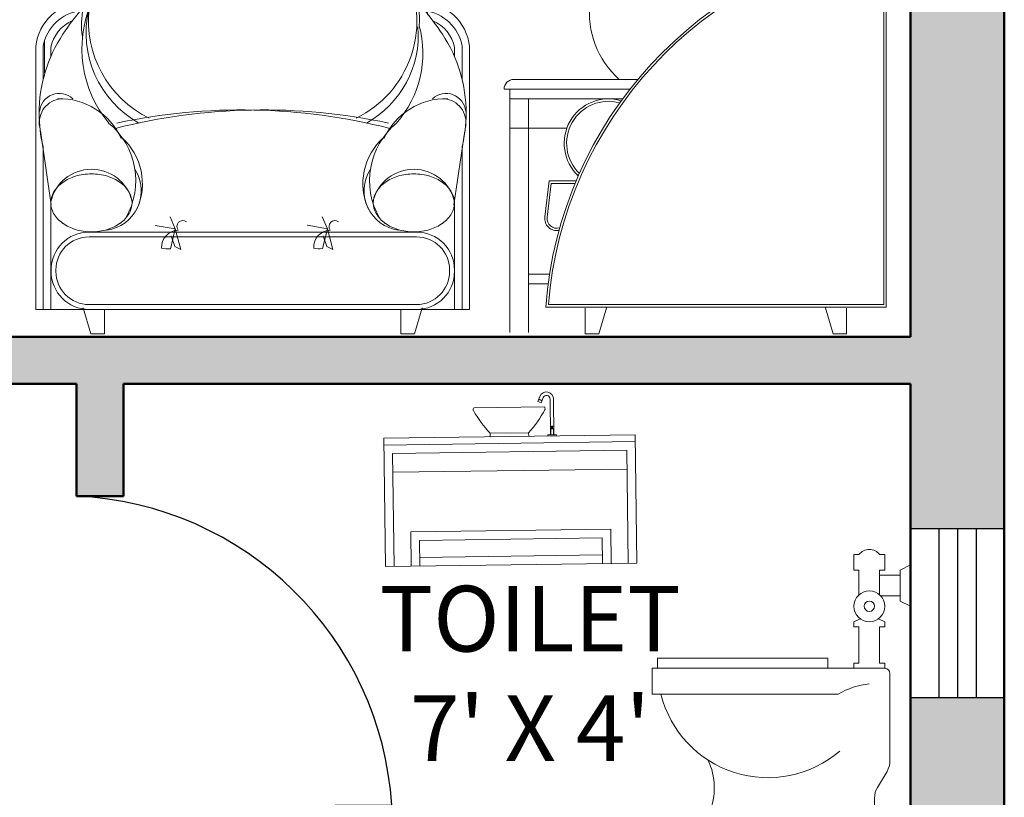
# Model space of a CAD drawing. Units: inches. Extents: x 1771 to 3025, y 319 to 889.
# Tile 21 of 35: x 2456 to 2561, y 621 to 703. Entities that reach past the tile are written whole.
import ezdxf

# ---------------------------------------------------------------- set-up
doc = ezdxf.new("R2010")
doc.units = ezdxf.units.IN
doc.header["$MEASUREMENT"] = 0
doc.set_wipeout_variables(frame=1)
for name, color, linetype, lineweight in [('A-AREA-IDEN', 241, 'Continuous', 25), ('A-DOOR', 4, 'Continuous', 25), ('A-FLOR-FIXT', 8, 'Continuous', 18), ('A-FURN', 8, 'Continuous', 18), ('A-GLAZ', 40, 'Continuous', 25), ('A-WALL', 7, 'Continuous', 50), ('A-WALL-PATT', 254, 'Continuous', 13)]:
    doc.layers.add(name, color=color, linetype=linetype, lineweight=lineweight)
doc.styles.get("Standard").update_dxf_attribs({"font": 'arial.ttf'})

# ---------------------------------------------------------------- blocks, each defined once
blk = doc.blocks.new('A$C425441F1')
for points in [[(1639.3, 0), (1667.3, 0), (1667.3, 55.3), (1748.6, 55.3), (1748.6, 807.4), (1761.1, 860.7), (1735.7, 880.7), (1703.4, 883.3), (1675.8, 879.6), (1656.2, 873.5), (1635.2, 863.3), (1619.6, 852.6), (1605.1, 839.5), (1596.7, 829.9), (1583.2, 810), (1573.2, 788.1), (1567.6, 767.7), (1566.5, 761.6), (1541.6, 750.9), (1510.7, 736.6), (1488.3, 725.3), (1464.5, 712.2), (1433.4, 693.6), (1409.1, 677.8), (1389.7, 664.2), (1388.2, 683.8), (1383.3, 700), (1376.2, 712), (1365.5, 723.2), (1352, 731.8), (1342.1, 735.4), (1331.7, 738.6), (1325, 742.7), (1317.7, 750.9), (1314.2, 758.8), (1312.9, 767.9), (1315.6, 780.8), (1321.1, 788.9), (1323.4, 793.7), (1323.6, 797.2), (1323.1, 800), (1320.5, 804.5), (1317.8, 806.7), (1317.8, 807.1), (1478.8, 807.1), (1345.8, 1080.7), (1177.3, 1080.7), (1044.3, 807.1), (1211.1, 807.1), (1211.1, 806.7), (1207.8, 803.9), (1205.8, 800.4), (1205.1, 796.3), (1207.6, 788.9), (1211.4, 783.4), (1213.5, 778.7), (1215.3, 769.8), (1215.1, 763.9), (1214.1, 759), (1208.8, 748.5), (1201.9, 741.7), (1195.3, 738), (1185.9, 735.4), (1176, 731.7), (1166.8, 726.4), (1159.9, 720.8), (1156.8, 717.7), (1149.3, 708.1), (1145.7, 701.6), (1143.6, 696.9), (1138.7, 669.7), (1138.7, 651.6), (1140.7, 631.8), (1142.6, 621.6), (1148.5, 600.5), (1162.8, 569), (1176.9, 547.8), (1188.6, 534.2), (1200, 523), (983, 523), (977.7, 522.3), (971.8, 519.6), (965.5, 512.8), (963.3, 506.8), (963, 503), (974.8, 503), (974.8, 3), (1013, 3), (1013, 103), (1053.6, 103), (1052.7, 96.1), (1051.6, 86.5), (1049.3, 63.6), (1048.6, 55.3), (1130.1, 55.3), (1130.1, 0), (1157.9, 0), (1174.1, 55.3), (1623.1, 55.6)], [(778.6, 0), (750.6, 0), (750.6, 50.4), (141.4, 50.4), (141.4, 0), (113.4, 0), (98.1, 50.4), (0, 50.4), (0, 590.4), (3.6, 609.1), (14.7, 633.7), (36.6, 658.7), (60.6, 673.3), (86.6, 680.5), (100.5, 681.5), (107.8, 698), (118.3, 717), (136.4, 751.3), (159.1, 779.5), (188.4, 803.6), (213.2, 817.4), (239.4, 827.1), (258.7, 831.4), (276, 833.4), (301.1, 842.1), (332.2, 850.9), (368.4, 858.6), (403.3, 863.5), (432.7, 865.8), (472.6, 866.2), (499.3, 864.8), (525, 862.1), (551.9, 857.9), (572.9, 853.6), (591.1, 849.1), (612.6, 842.8), (648, 830.4), (661.5, 823.7), (679.5, 815.2), (707.5, 798.2), (726.7, 783.3), (755.4, 754.4), (773.7, 729.8), (788.1, 704.9), (796.6, 686.1), (798.5, 681.2), (818, 677.9), (833.5, 672.3), (851.7, 661.6), (864.4, 650.3), (878.3, 632.1), (887.5, 611.7), (891.4, 595.2), (892, 590.4), (892, 50.4), (793.9, 50.4)]]:
    blk.add_wipeout(points)
for p, q in [((1044.3, 807.1), (1177.3, 1080.7)), ((1177.3, 1080.7), (1044.3, 807.1)), ((1177.3, 1080.7), (1345.8, 1080.7)), ((1345.8, 1080.7), (1177.3, 1080.7)), ((1345.8, 1080.7), (1478.8, 807.1)), ((1478.8, 807.1), (1345.8, 1080.7)), ((1188.8, 1068), (1069.3, 827.4)), ((1201.1, 1068), (1081.6, 827.4)), ((1211.2, 1068), (1091.7, 827.4)), ((1223.5, 1068), (1104, 827.4)), ((1230.5, 1068), (1110.9, 827.4)), ((1242.8, 1068), (1123.2, 827.4)), ((1171, 1067.8), (1351.9, 1067.8)), ((1299.6, 1068), (1419.2, 827.4)), ((1311.9, 1068), (1431.5, 827.4)), ((1322, 1068), (1441.5, 827.4)), ((1334.3, 1068), (1453.8, 827.4)), ((1733.6, 876.1), (1755.5, 858.7)), ((1735.7, 880.7), (1761.1, 860.7)), ((1744.1, 810.1), (1755.5, 858.7)), ((1748.6, 807.4), (1761.1, 860.7)), ((1053.8, 826.7), (1469.3, 826.7)), ((1478.8, 807.1), (1044.3, 807.1)), ((1044.3, 807.1), (1478.8, 807.1)), ((1205.6, 800), (1323.1, 800)), ((1211, 806.7), (1317.8, 806.7)), ((1743.6, 60.3), (1743.6, 805)), ((1748.6, 55.3), (1748.6, 807.4)), ((0, 590.4), (0, 50.4)), ((15, 591.1), (15, 521.6)), ((18.2, 603.6), (18.2, 536.8)), ((31, 569.9), (31, 588.4)), ((861, 569.9), (861, 588.4)), ((877, 591.1), (877, 521.6)), ((892, 590.4), (892, 50.4)), ((1238.2, 523), (983, 523)), ((1222, 503), (963, 503)), ((974.8, 3), (974.8, 503)), ((1206.8, 483), (974.8, 483)), ((1013, 3), (1013, 483)), ((10, 417.4), (32, 265.4)), ((882, 417.4), (860, 265.4)), ((1092.2, 423), (974.8, 423)), ((15, 385.1), (15, 50.4)), ((877, 385.1), (877, 50.4)), ((1055.6, 314.3), (1046.6, 240.3)), ((1060.1, 309.3), (1051.6, 239.7)), ((1111.1, 314.3), (1055.6, 314.3)), ((1109, 309.3), (1060.1, 309.3)), ((31, 50.4), (31, 272.3)), ((861, 50.4), (861, 272.3)), ((245.5, 223.1), (286.9, 216)), ((276.3, 240.8), (286.9, 216)), ((558.4, 223.2), (599.9, 216.1)), ((589.2, 240.9), (599.9, 216.1)), ((108.8, 209.4), (790.1, 209.4)), ((109.6, 209.4), (783, 209.4)), ((286.9, 216), (276.9, 175.2)), ((286.9, 216), (298.3, 173.5)), ((599.9, 216.1), (589.8, 175.3)), ((599.9, 216.1), (611.2, 173.6)), ((109.6, 199.4), (783, 199.4)), ((285.7, 179.9), (278.3, 201.7)), ((598.7, 180), (591.2, 201.8)), ((298.3, 173.5), (285.7, 179.9)), ((611.2, 173.6), (598.7, 180)), ((31.6, 128.4), (31.6, 131.4)), ((41.6, 128.4), (41.6, 131.4)), ((851, 131.4), (851, 128.4)), ((861, 131.4), (861, 128.4)), ((1056.5, 123), (1013, 123)), ((1053.6, 103), (1013, 103)), ((0, 50.4), (892, 50.4)), ((113.4, 0), (97.2, 53.4)), ((783, 60.4), (109.6, 60.4)), ((783, 50.4), (109.6, 50.4)), ((141.4, 50.4), (141.4, 0)), ((750.6, 50.4), (750.6, 0)), ((778.6, 0), (794.8, 53.4)), ((1048.6, 55.3), (1748.6, 55.3)), ((1054, 60.3), (1743.6, 60.3)), ((1129.9, 52.6), (1129.9, 0)), ((1157.9, 0), (1174.2, 55.6)), ((1639.3, 0), (1623.1, 55.6)), ((1667.3, 52.6), (1667.3, 0)), ((141.4, 0), (113.4, 0)), ((750.6, 0), (778.6, 0)), ((1129.9, 0), (1157.9, 0)), ((1667.3, 0), (1639.3, 0))]:
    blk.add_line(p, q)
for centre, radius, start, end in [((1708.4, 739.8), 143.6, 79.0486, 171.2543), ((1708.4, 739.8), 138.6, 79.5487, 170.0411), ((458.1, 348.7), 517.8, 68.4843, 110.5916), ((458.1, 348.7), 512.8, 68.4843, 110.5916), ((289.3, 651.4), 182.6, 93.9855, 176.965), ((563, 591.9), 251.9, 14.3659, 71.2419), ((289.3, 651.4), 177.6, 93.9855, 170.8791), ((563, 591.9), 246.9, 17.5917, 71.2419), ((1873.1, -6.5), 826.8, 98.9741, 175.711), ((1873.1, -6.5), 821.8, 99.0642, 175.3352), ((1217.2, 796.3), 12.1, 120.8914, 217.6223), ((1345.2, 767.9), 32.3, 135.1029, 257.7671), ((1311.5, 796.3), 12.1, 322.3777, 59.1086), ((1183, 767.9), 32.3, 282.2329, 40.4775), ((560.7, 643.7), 223.1, 296.1387, 23.9967), ((1203.5, 673.6), 64.2, 102.2329, 173.5671), ((1324.7, 673.6), 64.2, 6.4329, 77.7671), ((242.1, 635.9), 148, 144.2704, 189.5276), ((512.5, 645.7), 276.4, 357.4515, 12.4082), ((100.5, 580.5), 100.9, 89.5113, 174.4069), ((508.9, 316.7), 542.9, 139.0716, 146.5815), ((333.5, 586), 238.7, 156.9166, 219.7497), ((331.3, 643.7), 223.1, 173.6107, 243.8613), ((791.5, 580.5), 100.9, 5.5931, 89.1441), ((1322.1, 660.2), 183.7, 173.5671, 228.321), ((1206.1, 660.2), 183.7, 1.2452, 6.4329), ((104.5, 574.5), 91, 97.7735, 169.4907), ((316.8, 619.2), 213.4, 167.2983, 240.5749), ((383.1, 316.7), 542.9, 33.4185, 40.1113), ((787.5, 574.5), 91, 10.5093, 82.2265), ((104.5, 574.5), 74.8, 113.0142, 169.2704), ((579.4, 614.6), 207.2, 299.0365, 4.5654), ((578.1, 577), 217.9, 318.7723, 15.0106), ((787.5, 574.5), 74.8, 10.7296, 66.9858), ((301.8, 453.4), 294.8, 146.5815, 180), ((590.2, 453.4), 294.8, 0, 33.4185), ((983, 503), 20, 90, 180), ((48.3, 453.8), 40.5, 46.9039, 174.9451), ((843.7, 453.8), 40.5, 5.0549, 133.0961), ((56.7, 434.2), 49.4, 95.5103, 189.1585), ((49, 344.1), 139.3, 24.2628, 91.6479), ((843, 344.1), 139.3, 88.3521, 155.7372), ((835.3, 434.2), 49.4, 350.8415, 84.4897), ((1177.9, 391.7), 91.3, 73.3794, 227.0029), ((1177.9, 391.7), 86.3, 74.5383, 225.8439), ((301.8, 453.4), 294.8, 180, 193.379), ((468.1, -775.2), 1235.6, 77.9993, 104.2473), ((423.9, -775.2), 1235.6, 75.7527, 102.0007), ((590.2, 453.4), 294.8, 346.621, 0), ((52.4, 315.2), 153.2, 329.9033, 50.4478), ((839.6, 315.2), 153.2, 129.5522, 210.0967), ((92.5, 308.8), 126.8, 335.5815, 48.2351), ((799.5, 308.8), 126.8, 131.7649, 204.4185), ((114.7, 252.6), 85.8, 14.0074, 167.3648), ((106.2, 240.2), 87.4, 106.4444, 125.4727), ((114.5, 212.1), 116.8, 90, 106.4444), ((114.5, 212.1), 116.8, 73.5556, 90), ((135.5, 294.2), 81.5, 277.3995, 32.8179), ((122.8, 240.2), 87.4, 54.5273, 73.5556), ((756.5, 294.2), 81.5, 147.1821, 262.6005), ((777.3, 252.6), 85.8, 12.6352, 165.9926), ((769.2, 240.2), 87.4, 106.4444, 125.4727), ((777.5, 212.1), 116.8, 90, 106.4444), ((777.5, 212.1), 116.8, 73.5556, 90), ((785.8, 240.2), 87.4, 54.5273, 73.5556), ((93.5, 258.1), 65.5, 125.4727, 149.8309), ((135.5, 258.1), 65.5, 30.1691, 54.5273), ((756.5, 258.1), 65.5, 125.4727, 149.8309), ((798.5, 258.1), 65.5, 30.1691, 54.5273), ((74.1, 269.4), 43.1, 149.8309, 180), ((154.9, 269.4), 43.1, 0, 30.1691), ((737.1, 269.4), 43.1, 149.8309, 180), ((817.9, 269.4), 43.1, 0, 30.1691), ((74.1, 269.4), 43.1, 180, 210.1691), ((154.9, 269.4), 43.1, 329.8309, 0), ((737.1, 269.4), 43.1, 180, 210.1691), ((817.9, 269.4), 43.1, 329.8309, 0), ((93.5, 280.6), 65.5, 210.1691, 234.5273), ((135.5, 280.6), 65.5, 305.4727, 329.8309), ((756.5, 280.6), 65.5, 210.1691, 234.5273), ((798.5, 280.6), 65.5, 305.4727, 329.8309), ((106.2, 298.5), 87.4, 234.5273, 253.5556), ((122.8, 298.5), 87.4, 286.4444, 305.4727), ((302.4, 220.7), 12.2, 53.3958, 216.551), ((615.4, 220.8), 12.2, 53.3958, 216.551), ((769.2, 298.5), 87.4, 234.5273, 253.5556), ((785.8, 298.5), 87.4, 286.4444, 305.4727), ((1071.6, 237.3), 25.1, 173.0657, 279.7438), ((1071.6, 237.3), 20.1, 173.0657, 286.6808), ((109.6, 131.4), 78, 90, 180), ((114.5, 326.6), 116.8, 253.5556, 270), ((114.5, 326.6), 116.8, 270, 286.4444), ((294.4, 177.6), 35.9, 92.8846, 181.9), ((607.4, 177.7), 35.9, 92.8846, 181.9), ((777.5, 326.6), 116.8, 253.5556, 270), ((777.5, 326.6), 116.8, 270, 286.4444), ((783, 131.4), 78, 0, 90), ((109.6, 131.4), 68, 90, 180), ((783, 131.4), 68, 0, 90), ((271.5, 234.5), 59.6, 257.4358, 275.1883), ((584.4, 234.6), 59.6, 257.4358, 275.1883), ((109.6, 128.4), 78, 180, 270), ((109.6, 128.4), 68, 180, 270), ((783, 128.4), 68, 270, 0), ((783, 128.4), 78, 270, 0)]:
    blk.add_arc(centre, radius, start, end)
blk = doc.blocks.new('A$C062C426B')
for p, q in [((0.4867, 0.6739, -0.3429), (0.4867, 0.6365, -0.3429)), ((0.4992, 0.6739, -0.3429), (0.4867, 0.6739, -0.3429)), ((0.5616, 0.6739, -0.3429), (0.5491, 0.6739, -0.3429)), ((0.5616, 0.6365, -0.3429), (0.5616, 0.6739, -0.3429)), ((0.624, 0.649, -0.3429), (0.599, 0.6365, -0.3429)), ((0.624, 0.5491, -0.3429), (0.624, 0.649, -0.3429)), ((0.4867, 0.6365, -0.3429), (0.4992, 0.6365, -0.3429)), ((0.4992, 0.6365, -0.3429), (0.4992, 0.577, -0.3429)), ((0.5491, 0.6365, -0.3429), (0.5616, 0.6365, -0.3429)), ((0.5491, 0.577, -0.3429), (0.5491, 0.6365, -0.3429)), ((0.599, 0.624, -0.3429), (0.5491, 0.624, -0.3429)), ((0.599, 0.6365, -0.3429), (0.599, 0.5616, -0.3429)), ((0.5521, 0.5741, -0.3429), (0.599, 0.5741, -0.3429)), ((0.599, 0.5616, -0.3429), (0.624, 0.5491, -0.3429)), ((0.4867, 0.5117, -0.3429), (0.5017, 0.5192, -0.3429)), ((0.4867, 0.4992, -0.3429), (0.4867, 0.5117, -0.3429)), ((0.5616, 0.5117, -0.3429), (0.5466, 0.5192, -0.3429)), ((0.5616, 0.4992, -0.3429), (0.5616, 0.5117, -0.3429)), ((0.4867, 0.4992, -0.3429), (0.4992, 0.4992, -0.3429)), ((0.4992, 0.4118, -0.3429), (0.4992, 0.4992, -0.3429)), ((0.5491, 0.4118, -0.3429), (0.5491, 0.4992, -0.3429)), ((0.5491, 0.4992, -0.3429), (0.5616, 0.4992, -0.3429)), ((0.4243, 0.4243, -0.3429), (0.0125, 0.4243, -0.3429)), ((0.0125, 0.4243, -0.3429), (0.0125, 0.3994, -0.3429)), ((0.4243, 0.3994, -0.3429), (0.4243, 0.4243, -0.3429)), ((0.4992, 0.4118, -0.3429), (0.4867, 0.4118, -0.3429)), ((0.4867, 0.4118, -0.3429), (0.4867, 0.3994, -0.3429)), ((0.5616, 0.4118, -0.3429), (0.5491, 0.4118, -0.3429)), ((0.5616, 0.3994, -0.3429), (0.5616, 0.4118, -0.3429)), ((0.5616, 0.3994, -0.3429), (0, 0.3994, -0.3429)), ((0, 0.3994, -0.3429), (0, 0.337, -0.3429)), ((0.5741, 0.3869, -0.3429), (0.5741, 0.1761, -0.3429)), ((0, 0.337, -0.3429), (0.4493, 0.337, -0.3429)), ((0.567, 0.1504, -0.3429), (0.5438, 0.1117, -0.3429)), ((0.5366, 0.086, -0.3429), (0.5366, 0, -0.3429)), ((0.5366, 0.0499, -0.3429), (0.1373, 0.0499, -0.3429)), ((0.1373, 0.0499, -0.3429), (0.1373, 0.0374, -0.3429)), ((0.5366, 0.0374, -0.3429), (0.1248, 0.0374, -0.3429)), ((0.1248, 0.0374, -0.3429), (0.1248, 0, -0.3429))]:
    blk.add_line(p, q)
for radius in [0.0374, 0.0125]:
    blk.add_circle((0.5242, 0.5491, -0.3429), radius)
for centre, radius, start, end in [((0.5242, 0.6552, -0.3429), 0.0312, 36.8699, 143.1301), ((0.5616, 0.3869, -0.3429), 0.0125, 0, 90), ((0.5429, 0.181, -0.3429), 0.1819, 95.9061, 120.9638), ((0.2791, 0.4017, -0.3429), 0.2664, 194.0552, 310.7015), ((-0.0044, 0.1107, -0.3429), 0.1542, 336.7818, 25.8778), ((0.5242, 0.1761, -0.3429), 0.0499, 329.0362, 0), ((0.5866, 0.086, -0.3429), 0.0499, 149.0362, 180)]:
    blk.add_arc(centre, radius, start, end)
blk = doc.blocks.new('A$C127E6D2A')
for p, q in [((0.904, 0.9521), (0.9161, 0.9819)), ((0.9226, 0.9446), (0.904, 0.9521)), ((0.9275, 0.9563), (0.9088, 0.9639)), ((0.9282, 0.9582), (0.9095, 0.9657)), ((0.9226, 0.9446), (0.9346, 0.9744)), ((0.975, 0.9647), (0.975, 0.756)), ((0.995, 0.964), (0.995, 0.756)), ((0.525, 0.915), (0.525, 0.9063)), ((0.525, 0.915), (0.525, 0.9063)), ((0.94, 0.92), (0.53, 0.92)), ((0.945, 0.915), (0.945, 0.9063)), ((1.47, 0.75), (0, 0.75)), ((0, 0.75), (0, 0)), ((0.6225, 0.77), (0.6225, 0.75)), ((0.8475, 0.77), (0.6225, 0.77)), ((0.8475, 0.75), (0.6225, 0.75)), ((0.8475, 0.77), (0.8475, 0.75)), ((0.96, 0.756), (0.96, 0.75)), ((0.96, 0.756), (1.01, 0.756)), ((0.9925, 0.7905), (0.9775, 0.7905)), ((0.9775, 0.7905), (0.9775, 0.756)), ((0.982, 0.8022), (0.982, 0.7905)), ((0.988, 0.8022), (0.988, 0.7905)), ((0.9925, 0.7905), (0.9925, 0.756)), ((1.01, 0.756), (1.01, 0.75)), ((1.47, 0), (1.47, 0.75)), ((1.47, 0.71), (0, 0.71)), ((0.05, 0.66), (0.05, 0)), ((1.42, 0.66), (0.05, 0.66)), ((1.42, 0), (1.42, 0.66)), ((0.05, 0.55), (1.42, 0.55)), ((1.32, 0.2), (0.15, 0.2)), ((0.15, 0.2), (0.15, 0)), ((1.32, 0), (1.32, 0.2)), ((1.27, 0.15), (0.2, 0.15)), ((0.2, 0.15), (0.2, 0)), ((1.27, 0), (1.27, 0.15)), ((0.2, 0.05), (1.27, 0.05)), ((0, 0), (1.47, 0))]:
    blk.add_line(p, q)
blk.add_circle((0.985, 0.804), 0.0035)
for centre, radius, start, end in [((0.9541, 0.9665), 0.041, 356.58807, 157.98673), ((0.9541, 0.9665), 0.021, 355.23192, 157.98673), ((0.53, 0.915), 0.005, 90, 180), ((0.53, 0.9063), 0.005, 180, 209.45502), ((1.1676, 1.2664), 0.7372, 209.45502, 222.32259), ((0.3024, 1.2664), 0.7372, 317.67741, 330.54498), ((0.94, 0.915), 0.005, 0, 90), ((0.94, 0.9063), 0.005, 330.54498, 0)]:
    blk.add_arc(centre, radius, start, end)
blk = doc.blocks.new('DOOR-35')
blk.add_lwpolyline([(35.88, 36.19), (32.96, 36.3), (33.16, 0), (36, 0.05)], close=True)
blk.add_arc((35.23, 1.11), 35.26, 93.6879, 177.4925)
blk = doc.blocks.new('WIN-18')
for p, q in [((0, 0), (0, 10)), ((18, 0), (18, 10)), ((0, 7), (18, 7)), ((0, 5), (18, 5)), ((0, 3), (18, 3))]:
    blk.add_line(p, q)

msp = doc.modelspace()

# ---------------------------------------------------------------- hatches: boundary and pattern name
at = {"layer": 'A-WALL-PATT'}
h = msp.add_hatch(color=256, dxfattribs=at)
h.dxf.hatch_style = 1
h.paths.add_polyline_path([(2407.16, 878.63), (2429.21, 878.63), (2429.21, 888.63), (2379.16, 888.63), (2379.16, 878.63), (2402.16, 878.63), (2402.16, 830.63), (2407.16, 830.63)])
h.paths.add_polyline_path([(2520.11, 888.63), (2477.21, 888.63), (2477.21, 878.63), (2498.16, 878.63), (2498.16, 794.63), (2402.16, 794.63), (2402.16, 758.63), (2402.16, 664.63), (2407.16, 664.63), (2407.16, 712), (2407.16, 789.63), (2515.16, 789.63), (2515.16, 794.63), (2503.16, 794.63), (2503.16, 878.63), (2520.11, 878.63)])
h.paths.add_polyline_path([(2561.16, 888.63), (2538.11, 888.63), (2538.11, 878.63), (2551.16, 878.63), (2551.16, 789.63), (2551.16, 768.61), (2561.16, 768.61)])
h.paths.add_polyline_path([(2561.16, 720.61), (2551.16, 720.61), (2551.16, 669.63), (2443.16, 669.63), (2443.16, 664.63), (2462.16, 664.63), (2462.16, 652.63), (2467.16, 652.63), (2467.16, 664.63), (2551.16, 664.63), (2551.16, 649.17), (2561.16, 649.17)])
h.paths.add_polyline_path([(2561.16, 631.17), (2551.16, 631.17), (2551.16, 616.63), (2462.16, 616.63), (2443.16, 616.63), (2443.16, 611.63), (2551.16, 611.63), (2551.16, 581.11), (2561.16, 581.11)])
h.paths.add_polyline_path([(2561.16, 533.11), (2551.16, 533.11), (2551.16, 479.63), (2407.16, 479.63), (2407.16, 616.63), (2397.16, 616.63), (2397.16, 543.63), (2306.16, 543.63), (2306.16, 533.63), (2397.16, 533.63), (2397.16, 469.63), (2551.16, 469.63), (2551.16, 452.76), (2561.16, 452.76)])
h.paths.add_polyline_path([(2561.16, 404.76), (2551.16, 404.76), (2551.16, 393.63), (2397.16, 393.63), (2397.16, 383.63), (2561.16, 383.63)])
h.paths.add_polyline_path([(2270.16, 642.58), (2260.16, 642.58), (2260.16, 533.63), (2270.16, 533.63)])
h.paths.add_polyline_path([(2270.16, 753.63), (2366.16, 753.63), (2366.16, 758.63), (2270.16, 758.63), (2270.16, 842.59, -0.008336), (2268.86, 842.63), (2260.16, 842.63), (2260.16, 690.58), (2270.16, 690.58)])
h.paths.add_polyline_path([(2331.16, 888.63), (2260.16, 888.63), (2260.16, 878.63), (2331.16, 878.63)])

# ---------------------------------------------------------------- linework, layer by layer
at = {"layer": 'A-WALL'}
for p, q in [((2561.16, 383.63), (2561.16, 888.43)), ((2551.16, 669.63), (2551.16, 789.63)), ((2551.16, 669.63), (2443.16, 669.63)), ((2462.16, 664.63), (2443.16, 664.63)), ((2462.16, 652.63), (2462.16, 664.63)), ((2467.16, 652.63), (2467.16, 664.63)), ((2551.16, 664.63), (2467.16, 664.63)), ((2551.16, 616.63), (2551.16, 664.63)), ((2467.16, 652.63), (2462.16, 652.63))]:
    msp.add_line(p, q, dxfattribs=at)

# ---------------------------------------------------------------- block references
at = {"layer": 'A-DOOR', "rotation": 269.9999999999959}
msp.add_blockref('DOOR-35', (2459.5, 652.63), dxfattribs=at)
at = {"layer": 'A-FLOR-FIXT', "xscale": 18.24536006826809, "yscale": 18.24536006826809, "zscale": 18.24536006826809, "rotation": 0.7699301504024306}
msp.add_blockref('A$C127E6D2A', (2495.13, 645.14, 15.15), dxfattribs=at)
at = {"layer": 'A-FLOR-FIXT', "xscale": 44.17762020618112, "yscale": 44.17762020618112, "zscale": 44.17762020618112}
msp.add_blockref('A$C062C426B', (2523.6, 616.63, 15.15), dxfattribs=at)
at = {"layer": 'A-GLAZ', "rotation": 269.9999999999966}
msp.add_blockref('WIN-18', (2551.16, 649.17), dxfattribs=at)

# ---------------------------------------------------------------- texts
at = {"layer": 'A-AREA-IDEN', "insert": (2467.84, 643.07), "char_height": 7, "attachment_point": 1}
msp.add_mtext_dynamic_manual_height_columns("\\pxqc;TOILET \\P7' X 4'", width=85.4611, gutter_width=1, heights=[0], dxfattribs=at)

# ---------------------------------------------------------------- next in the draw order: block references
at = {"layer": 'A-FURN', "xscale": 0.0519011286993662, "yscale": 0.0519011286993662, "zscale": 0.0519011286993662}
msp.add_blockref('A$C425441F1', (2457.8, 669.94), dxfattribs=at)

doc.saveas('drawing.dxf')
